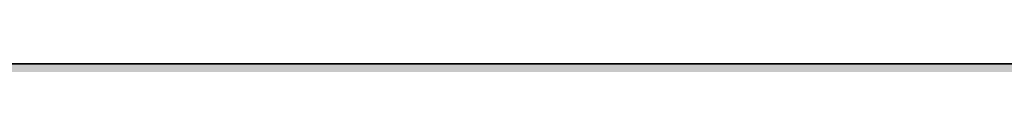
# Model space of a CAD drawing. Units: inches. Extents: x 2083 to 3317, y 1141 to 2115.
# Tile 73 of 256: x 2238.294 to 2242.452, y 1477.761 to 1477.761. Entities that reach past the tile are written whole.
import ezdxf

# ---------------------------------------------------------------- set-up
doc = ezdxf.new("R2010")
doc.units = ezdxf.units.IN
doc.layers.add('A-ANNO-DIMS', color=2, linetype='Continuous', lineweight=18)
doc.layers.add('A-WALL', color=7, linetype='Continuous', lineweight=35)
doc.layers.add('A-WALL-PATT', color=251, linetype='Continuous', lineweight=13, true_color=0x636466)
doc.styles.get("Standard").update_dxf_attribs({"font": 'arial.ttf'})
doc.dimstyles.new('ISO-25', dxfattribs={"dimtxt": 12, "dimasz": 12, "dimexe": 1.25, "dimexo": 0.625, "dimtad": 1, "dimlunit": 3, "dimtxsty": 'Standard', "dimcen": 2.5, "dimadec": 0, "dimazin": 0, "dimtfac": 1, "dimtmove": 0, "dimatfit": 3, "dimfxl": 1, "dimarcsym": 0})

# ---------------------------------------------------------------- blocks, each defined once
blk = doc.blocks.new('*D30')
at = {"layer": 'A-ANNO-DIMS', "color": 0, "lineweight": -2, "transparency": 16777216}
for p, q in [((2240.0179, 1445.2738), (2240.0179, 1448.0455)), ((2254.3293, 1445.2738), (2254.3293, 1448.0455)), ((2228.0179, 1446.7955), (2216.0179, 1446.7955)), ((2240.0179, 1446.7955), (2254.3293, 1446.7955)), ((2266.3293, 1446.7955), (2413.7649, 1446.7955))]:
    blk.add_line(p, q, dxfattribs=at)
at = {"layer": 'A-ANNO-DIMS', "color": 0, "transparency": 16777216}
for points in [[(2228.0179, 1448.7955), (2228.0179, 1444.7955), (2240.0179, 1446.7955)], [(2266.3293, 1448.7955), (2266.3293, 1444.7955), (2254.3293, 1446.7955)]]:
    blk.add_solid(points, dxfattribs=at)
at = {"layer": 'Defpoints', "color": 0, "transparency": 16777216}
for p in [(2254.3293, 1446.7955), (2240.0179, 1444.6488), (2254.3293, 1444.6488)]:
    blk.add_point(p, dxfattribs=at)
at = {"layer": 'A-ANNO-DIMS', "color": 0, "transparency": 16777216, "insert": (2346.0471, 1453.6252), "char_height": 12, "attachment_point": 5}
blk.add_mtext('WC 1\'-2 1/2" TYP.', dxfattribs=at)
blk = doc.blocks.new('*D31')
at = {"layer": 'A-ANNO-DIMS', "color": 0, "lineweight": -2, "transparency": 16777216}
for p, q in [((2237.8711, 1456.6488), (2237.8711, 1541.9152)), ((2239.3929, 1444.6488), (2236.6211, 1444.6488)), ((2237.8711, 1431.5475), (2237.8711, 1444.6488)), ((2239.3929, 1431.5475), (2236.6211, 1431.5475)), ((2237.8711, 1419.5475), (2237.8711, 1407.5475))]:
    blk.add_line(p, q, dxfattribs=at)
at = {"layer": 'A-ANNO-DIMS', "color": 0, "transparency": 16777216}
for points in [[(2235.8711, 1456.6488), (2239.8711, 1456.6488), (2237.8711, 1444.6488)], [(2235.8711, 1419.5475), (2239.8711, 1419.5475), (2237.8711, 1431.5475)]]:
    blk.add_solid(points, dxfattribs=at)
at = {"layer": 'Defpoints', "color": 0, "transparency": 16777216}
for p in [(2237.8711, 1444.6488), (2240.0179, 1444.6488), (2240.0179, 1431.5475)]:
    blk.add_point(p, dxfattribs=at)
at = {"layer": 'A-ANNO-DIMS', "color": 0, "transparency": 16777216, "insert": (2231.2175, 1505.282), "char_height": 12, "attachment_point": 5, "rotation": 90}
blk.add_mtext('1\'-1" TYP.', dxfattribs=at)
blk = doc.blocks.new('*D45')
at = {"layer": 'A-ANNO-DIMS', "color": 0, "lineweight": -2, "transparency": 16777216}
for p, q in [((2235.9598, 1478.3864), (2235.9598, 1531.3614)), ((2418.9598, 1478.3864), (2418.9598, 1531.3614)), ((2247.9598, 1530.1114), (2406.9598, 1530.1114))]:
    blk.add_line(p, q, dxfattribs=at)
at = {"layer": 'A-ANNO-DIMS', "color": 0, "transparency": 16777216}
for points in [[(2247.9598, 1532.1114), (2247.9598, 1528.1114), (2235.9598, 1530.1114)], [(2406.9598, 1532.1114), (2406.9598, 1528.1114), (2418.9598, 1530.1114)]]:
    blk.add_solid(points, dxfattribs=at)
at = {"layer": 'Defpoints', "color": 0, "transparency": 16777216}
for p in [(2418.9598, 1530.1114), (2235.9598, 1477.7614), (2418.9598, 1477.7614)]:
    blk.add_point(p, dxfattribs=at)
at = {"layer": 'A-ANNO-DIMS', "color": 0, "transparency": 16777216, "insert": (2327.4598, 1536.8673), "char_height": 12, "attachment_point": 5}
blk.add_mtext('15\'-3"', dxfattribs=at)
blk = doc.blocks.new('*D62')
at = {"layer": 'A-ANNO-DIMS', "color": 0, "lineweight": -2, "transparency": 16777216}
for p, q in [((2235.9598, 1469.3864), (2235.9598, 1522.3614)), ((2379.9598, 1469.3864), (2379.9598, 1522.3614)), ((2247.9598, 1521.1114), (2367.9598, 1521.1114))]:
    blk.add_line(p, q, dxfattribs=at)
at = {"layer": 'A-ANNO-DIMS', "color": 0, "transparency": 16777216}
for points in [[(2247.9598, 1523.1114), (2247.9598, 1519.1114), (2235.9598, 1521.1114)], [(2367.9598, 1523.1114), (2367.9598, 1519.1114), (2379.9598, 1521.1114)]]:
    blk.add_solid(points, dxfattribs=at)
at = {"layer": 'Defpoints', "color": 0, "transparency": 16777216}
for p in [(2379.9598, 1521.1114), (2235.9598, 1468.7614), (2379.9598, 1468.7614)]:
    blk.add_point(p, dxfattribs=at)
at = {"layer": 'A-ANNO-DIMS', "color": 0, "transparency": 16777216, "insert": (2307.9598, 1527.8632), "char_height": 12, "attachment_point": 5}
blk.add_mtext('12\'-0"', dxfattribs=at)

msp = doc.modelspace()

# ---------------------------------------------------------------- hatches: boundary and pattern name
at = {"layer": 'A-WALL-PATT'}
h = msp.add_hatch(color=256, dxfattribs=at)
h.dxf.hatch_style = 1
h.paths.add_polyline_path([(3126.9598, 2020.7614), (2748.9598, 2020.7614), (2604.9598, 2020.7614), (2226.9598, 2020.7614), (2226.9598, 1702.7614), (2466.9598, 1702.7614), (2466.9598, 1582.7614), (2418.9598, 1582.7614), (2418.9598, 1477.7614), (2226.9598, 1477.7614), (2226.9598, 1263.2614), (2544.9598, 1263.2614), (2544.9598, 1411.7614), (2604.9598, 1411.7614), (2685.9598, 1411.7614), (2685.9598, 1420.7614), (2604.9598, 1420.7614), (2604.9598, 1573.7614), (2604.9598, 1702.7614), (2604.9598, 2011.7614), (2748.9598, 2011.7614), (2748.9598, 1702.7614), (2862.9598, 1702.7614), (2862.9598, 1621.7614), (2871.9598, 1621.7614), (2871.9598, 1702.7614), (2883.9598, 1702.7614), (2883.9598, 1706.9395, -0.026459), (2883.9598, 1711.7614), (2757.9598, 1711.7614), (2757.9598, 1807.7614), (2787.9598, 1807.7614), (2787.9598, 1812.2614), (2757.9598, 1812.2614), (2757.9598, 2011.7614), (2877.9598, 2011.7614), (2877.9598, 1812.2614), (2847.9598, 1812.2614), (2847.9598, 1807.7614), (2889.8357, 1807.7614), (2889.8357, 1812.2614), (2882.4598, 1812.2614), (2882.4598, 2011.7614), (3117.9598, 2011.7614), (3117.9598, 1812.2614), (2937.8357, 1812.2614), (2937.8357, 1807.7614), (2995.7098, 1807.7614), (2995.7098, 1796.1177), (3000.2098, 1796.1177), (3000.2098, 1807.7614), (3117.9598, 1807.7614), (3117.9598, 1711.7614), (3000.2098, 1711.7614), (3000.2098, 1760.1177), (2998.5727, 1760.1177, -0.020711), (2995.7098, 1760.1177), (2995.7098, 1711.7614), (2931.9598, 1711.7614), (2931.9598, 1702.7614), (3126.9598, 1702.7614)])
h.paths.add_polyline_path([(2471.4598, 2011.7614), (2471.4598, 1810.0114), (2462.7169, 1810.0114), (2462.7169, 1805.5114), (2505.9598, 1805.5114), (2505.9598, 1810.0114), (2475.9598, 1810.0114), (2475.9598, 2011.7614), (2595.9598, 2011.7614), (2595.9598, 1810.0114), (2565.9598, 1810.0114), (2565.9598, 1805.5114), (2595.9598, 1805.5114), (2595.9598, 1711.7614), (2235.9598, 1711.7614), (2235.9598, 1805.5114), (2353.7098, 1805.5114), (2353.7098, 1796.0542), (2358.2098, 1796.0542), (2358.2098, 1805.5114), (2414.7169, 1805.5114), (2414.7169, 1810.0114), (2235.9598, 1810.0114), (2235.9598, 2011.7614)], flags=16)
h.paths.add_polyline_path([(2270.2047, 1994.61), (2270.2047, 1970.61), (2246.2047, 1970.61), (2246.2047, 1994.61)], flags=0)
edge = h.paths.add_edge_path(flags=0)
edge.add_ellipse((2332.0274, 1899.7982), major_axis=(-3.043, 3.043), ratio=0.168252, start_angle=-161.3322, end_angle=-156.3071, ccw=False)
edge.add_ellipse((2333.082, 1898.7435), major_axis=(-1.0546, 1.0546), ratio=0.453532, start_angle=-123.371, end_angle=-94.1591)
edge = h.paths.add_edge_path(flags=0)
edge.add_ellipse((2332.0274, 1968.8763), major_axis=(3.043, 3.043), ratio=0.168252, start_angle=18.6678, end_angle=23.6929)
edge.add_spline(control_points=[(2332.9256, 1970.6911), (2332.2268, 1970.3361), (2330.8937, 1969.6589), (2328.4131, 1970.9321), (2327.2039, 1967.7487), (2324.7096, 1969.9556), (2322.5328, 1967.0124), (2320.0128, 1971.2958), (2317.6803, 1968.1578), (2316.0405, 1967.102), (2315.4269, 1966.8096)], knot_values=[0, 0, 0, 0, 2.267059, 4.324559, 6.685584, 8.878641, 11.121502, 14.300359, 17.755284, 19.732645, 19.732645, 19.732645, 19.732645], degree=3, periodic=0)
edge.add_ellipse((2332.0274, 1968.8763), major_axis=(3.043, 3.043), ratio=0.168252, start_angle=18.6678, end_angle=23.6929, ccw=False)
edge.add_ellipse((2333.082, 1969.9309), major_axis=(1.0546, 1.0546), ratio=0.453532, start_angle=56.629, end_angle=85.8409, ccw=False)
edge = h.paths.add_edge_path(flags=0)
edge.add_spline(control_points=[(2296.4283, 1967.9879), (2293.6278, 1965.3363), (2287.7036, 1959.7271), (2299.7439, 1949.9957), (2294.5326, 1935.6685), (2290.5732, 1920.6035), (2293.3941, 1909.9737), (2296.1854, 1904.9665)], knot_values=[0.099185, 0.099185, 0.099185, 0.099185, 0.345301, 0.619822, 0.982653, 1.386093, 1.810555, 1.810555, 1.810555, 1.810555], degree=3, periodic=0)
edge.add_spline(control_points=[(2296.1854, 1904.9665), (2297.3836, 1902.6193), (2298.001, 1901.9493), (2298.553, 1901.4682)], knot_values=[0.006246, 0.006246, 0.006246, 0.006246, 0.055476, 0.055476, 0.055476, 0.055476], degree=3, periodic=0)
edge.add_spline(control_points=[(2298.553, 1901.4682), (2297.2586, 1900.9232), (2295.2253, 1900.2321), (2293.0602, 1900.6142), (2292.1014, 1900.7884), (2292.0896, 1900.7906)], knot_values=[0.312835, 0.312835, 0.312835, 0.312835, 0.40178, 0.474987, 0.475903, 0.475903, 0.475903, 0.475903], degree=3, periodic=0)
edge.add_arc((2292.7936, 1904.6641), 3.937, 215.4209, 259.6982, ccw=False)
edge.add_spline(control_points=[(2289.5853, 1902.3823), (2289.4767, 1902.5351), (2289.3685, 1902.688), (2289.2609, 1902.8412)], knot_values=[0.102872, 0.102872, 0.102872, 0.102872, 0.116896, 0.116896, 0.116896, 0.116896], degree=3, periodic=0)
edge.add_spline(control_points=[(2289.2609, 1902.8412), (2288.6866, 1902.5502), (2287.64, 1902.0199), (2285.8813, 1901.874), (2283.853, 1901.5044), (2281.72, 1899.7105), (2278.467, 1899.4929), (2276.1571, 1901.8832), (2272.259, 1899.8041), (2267.7776, 1901.8432), (2262.2439, 1900.184), (2257.4149, 1901.7821), (2254.3184, 1900.7261), (2253.1783, 1900.3373)], knot_values=[0, 0, 0, 0, 1.907977, 3.477176, 5.261074, 7.972851, 11.680248, 13.717921, 16.939592, 22.789562, 27.502503, 33.595215, 37.145618, 37.145618, 37.145618, 37.145618], degree=3, periodic=0)
edge.add_line((2253.1783, 1900.3373), (2250.2442, 1902.8412))
edge.add_line((2250.2442, 1902.8412), (2250.2442, 1965.8333))
edge.add_line((2250.2442, 1965.8333), (2253.1783, 1968.3371))
edge.add_spline(control_points=[(2253.1783, 1968.3371), (2254.3184, 1967.9483), (2257.4149, 1966.8924), (2262.2439, 1968.4904), (2267.7776, 1966.8313), (2271.5267, 1968.5372), (2273.8759, 1967.8283), (2274.2067, 1967.7276)], knot_values=[0, 0, 0, 0, 0.09018, 0.244935, 0.364644, 0.513233, 0.537855, 0.537855, 0.537855, 0.537855], degree=3, periodic=0)
edge.add_arc((2274.3529, 1963.7933), 3.937, 72.0511, 92.1279, ccw=False)
edge.add_arc((2281.2969, 1985.23), 18.5963, 252.05113, 288.56572)
edge.add_arc((2292.3167, 1956.0289), 12.6461, 71.02679, 113.77822, ccw=False)
edge = h.paths.add_edge_path(flags=0)
edge.add_spline(control_points=[(2274.8994, 1951.8562), (2275.0662, 1951.6166), (2275.2327, 1951.3766), (2275.398, 1951.1359)], knot_values=[1.409916, 1.409916, 1.409916, 1.409916, 1.43159, 1.43159, 1.43159, 1.43159], degree=3, periodic=0)
edge.add_spline(control_points=[(2275.398, 1951.1359), (2275.7921, 1950.5619), (2276.1792, 1949.9838), (2276.5455, 1949.3971)], knot_values=[1.358238, 1.358238, 1.358238, 1.358238, 1.409916, 1.409916, 1.409916, 1.409916], degree=3, periodic=0)
edge.add_line((2276.5455, 1949.3971), (2277.4373, 1947.8622))
edge.add_spline(control_points=[(2277.4373, 1947.8622), (2276.3038, 1945.6731), (2274.6397, 1942.4269), (2274.6316, 1938.0939), (2272.7991, 1930.8515), (2274.3564, 1943.897), (2275.9477, 1947.9234), (2276.5455, 1949.3971)], knot_values=[0.005632, 0.005632, 0.005632, 0.005632, 0.186014, 0.266002, 0.357087, 0.59639, 0.739732, 0.739732, 0.739732, 0.739732], degree=3, periodic=0)
edge.add_spline(control_points=[(2276.5455, 1949.3971), (2276.1792, 1949.9838), (2275.7921, 1950.5619), (2275.398, 1951.1359)], knot_values=[1.358238, 1.358238, 1.358238, 1.358238, 1.409916, 1.409916, 1.409916, 1.409916], degree=3, periodic=0)
edge.add_spline(control_points=[(2275.398, 1951.1359), (2274.9425, 1950.0805), (2274.2078, 1948.0253), (2273.9346, 1944.8515), (2272.4685, 1937.6275), (2273.4662, 1945.6965), (2274.7006, 1951.0595), (2274.8994, 1951.8562)], knot_values=[0.104364, 0.104364, 0.104364, 0.104364, 0.189636, 0.269624, 0.36071, 0.600013, 0.644622, 0.644622, 0.644622, 0.644622], degree=3, periodic=0)
h.paths.add_polyline_path([(2269.1675, 1963.1276, -0.357527), (2268.1706, 1960.9764, -0.092561), (2268.1706, 1939.4363, -0.357527), (2269.1675, 1937.2851, -0.357527), (2267.0163, 1938.282, -0.164785), (2254.6856, 1938.282, -0.357527), (2252.5344, 1937.2851, -0.357527), (2253.5313, 1939.4363, -0.092561), (2253.5313, 1960.9764, -0.357527), (2252.5344, 1963.1276, -0.357527), (2254.6856, 1962.1307, -0.164785), (2267.0163, 1962.1307, -0.357527)], flags=0)
h.paths.add_polyline_path([(2248.8741, 1967.8018), (2248.8741, 1957.0277), (2249.4578, 1957.0277), (2249.4578, 1911.6468), (2248.8741, 1911.6468), (2248.8741, 1900.8727), (2246.5119, 1900.8727, 0.197327), (2244.1497, 1902.4569), (2244.1497, 1966.2176, 0.197327), (2246.5119, 1967.8018)], flags=0)
h.paths.add_polyline_path([(2269.1675, 1931.3893, -0.357527), (2268.1706, 1929.2381, -0.092561), (2268.1706, 1907.6981, -0.357527), (2269.1675, 1905.5469, -0.357527), (2267.0163, 1906.5438, -0.164785), (2254.6856, 1906.5438, -0.357527), (2252.5344, 1905.5469, -0.357527), (2253.5313, 1907.6981, -0.092561), (2253.5313, 1929.2381, -0.357527), (2252.5344, 1931.3893, -0.357527), (2254.6856, 1930.3925, -0.164785), (2267.0163, 1930.3925, -0.357527)], flags=0)
edge = h.paths.add_edge_path(flags=0)
edge.add_spline(control_points=[(2276.1969, 1906.7237), (2276.1681, 1909.0289), (2276.114, 1913.3719), (2270.5984, 1924.925), (2273.9052, 1919.0128), (2275.9217, 1916.2621), (2275.4746, 1912.4021), (2277.2579, 1910.3806), (2276.696, 1908.225), (2276.6462, 1906.813), (2276.6178, 1906.0084)], knot_values=[0, 0, 0, 0, 8.61026, 16.221274, 18.843057, 23.804898, 27.440828, 29.356102, 31.203478, 33.650687, 33.650687, 33.650687, 33.650687], degree=3, periodic=0)
edge.add_spline(control_points=[(2276.6178, 1906.0084), (2276.6233, 1905.6241), (2276.4977, 1904.6287), (2275.4418, 1903.8547), (2274.9373, 1903.0804), (2274.8591, 1902.8412)], knot_values=[0.156488, 0.156488, 0.156488, 0.156488, 0.184398, 0.231376, 0.250598, 0.250598, 0.250598, 0.250598], degree=3, periodic=0)
edge.add_line((2274.8591, 1902.8412), (2276.506, 1902.8412))
edge.add_spline(control_points=[(2276.506, 1902.8412), (2276.7883, 1903.0849), (2277.6651, 1904.1252), (2278.2495, 1904.3407), (2277.6539, 1908.5274), (2278.1557, 1906.2278), (2278.1005, 1905.2859), (2278.8467, 1904.069), (2277.8568, 1903.4149), (2277.8742, 1902.991), (2277.9036, 1902.8412)], knot_values=[0.059574, 0.059574, 0.059574, 0.059574, 0.080753, 0.103741, 0.16972, 0.176036, 0.207137, 0.240474, 0.262341, 0.27366, 0.27366, 0.27366, 0.27366], degree=3, periodic=0)
edge.add_line((2277.9036, 1902.8412), (2280.0298, 1902.8412))
edge.add_spline(control_points=[(2280.0298, 1902.8412), (2279.8882, 1903.0884), (2279.4993, 1903.9816), (2280.1523, 1905.9393), (2278.1036, 1909.6578), (2279.7624, 1907.1853), (2280.3279, 1904.8749), (2280.4851, 1903.4896), (2281.4633, 1903.2494), (2281.7583, 1902.9365), (2281.834, 1902.8412)], knot_values=[0.013856, 0.013856, 0.013856, 0.013856, 0.034874, 0.088867, 0.107879, 0.126738, 0.158714, 0.193757, 0.217487, 0.226722, 0.226722, 0.226722, 0.226722], degree=3, periodic=0)
edge.add_spline(control_points=[(2281.834, 1902.8412), (2281.7875, 1902.8267), (2281.647, 1902.783), (2281.3955, 1902.8595), (2281.0881, 1902.9852), (2280.7207, 1903.0609), (2280.3335, 1903.0257), (2280.1248, 1902.8989), (2280.0298, 1902.8412)], knot_values=[0, 0, 0, 0, 0.14413, 0.435517, 0.749276, 1.153046, 1.548371, 1.878348, 1.878348, 1.878348, 1.878348], degree=3, periodic=0)
edge.add_line((2280.0298, 1902.8412), (2277.9036, 1902.8412))
edge.add_spline(control_points=[(2277.9036, 1902.8412), (2277.8929, 1902.7959), (2277.8654, 1902.6796), (2277.6075, 1902.6875), (2277.2741, 1902.8007), (2276.8379, 1902.6198), (2276.5838, 1902.7893), (2276.506, 1902.8412)], knot_values=[0, 0, 0, 0, 0.127189, 0.326199, 0.628009, 1.24357, 1.515331, 1.515331, 1.515331, 1.515331], degree=3, periodic=0)
edge.add_line((2276.506, 1902.8412), (2274.8591, 1902.8412))
edge.add_spline(control_points=[(2274.8591, 1902.8412), (2274.8144, 1902.8986), (2274.7251, 1903.0134), (2274.4935, 1903.119), (2274.2443, 1902.9605), (2273.9371, 1903.1849), (2273.614, 1902.9831), (2273.4083, 1902.883), (2273.3223, 1902.8412)], knot_values=[0, 0, 0, 0, 0.21843, 0.436957, 0.687977, 0.990379, 1.398396, 1.69185, 1.69185, 1.69185, 1.69185], degree=3, periodic=0)
edge.add_spline(control_points=[(2273.3223, 1902.8412), (2273.6167, 1903.4457), (2274.274, 1904.5383), (2276.0272, 1904.5737), (2276.207, 1906.5836), (2276.1969, 1906.7237)], knot_values=[0.012227, 0.012227, 0.012227, 0.012227, 0.059472, 0.106218, 0.134458, 0.134458, 0.134458, 0.134458], degree=3, periodic=0)
h.paths.add_polyline_path([(2270.7761, 1897.7898), (2270.7761, 1873.7898), (2246.7761, 1873.7898), (2246.7761, 1897.7898)], flags=0)
h.paths.add_polyline_path([(2353.7098, 1760.0051), (2353.7098, 1760.0542), (2358.2098, 1760.0542, -0.033729)], flags=0)
h.paths.add_polyline_path([(2321.8191, 1737.5292), (2341.9953, 1737.5292, -0.414214), (2343.2033, 1736.3212), (2343.2033, 1721.0206, -0.414214), (2341.9953, 1719.8127), (2321.8191, 1719.8127, -0.414214), (2320.6112, 1721.0206), (2320.6112, 1736.3212, -0.414214)], flags=0)
h.paths.add_polyline_path([(2324.235, 1736.3212), (2339.5794, 1736.3212, -0.414214), (2341.9953, 1733.9053), (2341.9953, 1725.4497, -0.414214), (2339.5794, 1723.0338), (2333.6806, 1723.0338), (2333.8453, 1722.0455, -0.870646), (2335.4254, 1721.8259, -0.767327), (2333.9227, 1721.4232), (2331.291, 1721.4232, -0.767327), (2329.7883, 1721.8259, -0.870646), (2331.3684, 1722.0455), (2331.5331, 1723.0338), (2324.235, 1723.0338, -0.414214), (2321.8191, 1725.4497), (2321.8191, 1733.9053, -0.414214)], flags=0)
h.paths.add_polyline_path([(2570.4838, 1928.6154), (2589.6838, 1928.6154), (2590.1688, 1928.6154), (2590.1688, 1904.9934), (2570.4838, 1904.9934)], flags=0)
h.paths.add_polyline_path([(2574.4473, 1927.2638, -1), (2572.8288, 1927.2638, -1)], flags=0)
h.paths.add_polyline_path([(2573.0899, 1926.9409), (2573.925, 1927.776), (2574.1477, 1927.5533), (2573.3126, 1926.7182)], flags=0)
h.paths.add_polyline_path([(2578.7791, 1919.7296, -1), (2571.5917, 1919.7296, -1)], flags=0)
h.paths.add_polyline_path([(2578.3854, 1919.7296, -1), (2571.9854, 1919.7296, -1)], flags=0)
h.paths.add_polyline_path([(2331.5958, 1729.4762, -1), (2333.618, 1729.4762, -1)], flags=0)
h.paths.add_polyline_path([(2578.0342, 1927.2638, -1), (2576.4157, 1927.2638, -1)], flags=0)
h.paths.add_polyline_path([(2576.6889, 1927.5311), (2576.9116, 1927.7538), (2577.7467, 1926.9186), (2577.524, 1926.6959)], flags=0)
h.paths.add_polyline_path([(2578.1391, 1909.8595, -1), (2572.2317, 1909.8595, -1)], flags=0)
h.paths.add_polyline_path([(2577.7454, 1909.8595, -1), (2572.6254, 1909.8595, -1)], flags=0)
h.paths.add_polyline_path([(2583.7977, 1927.2638, -1), (2582.1792, 1927.2638, -1)], flags=0)
h.paths.add_polyline_path([(2582.7186, 1927.7538), (2583.5538, 1926.9186), (2583.3311, 1926.6959), (2582.4959, 1927.5311)], flags=0)
h.paths.add_polyline_path([(2582.4959, 1927.5311), (2582.7186, 1927.7538), (2583.5538, 1926.9186), (2583.3311, 1926.6959)], flags=0)
h.paths.add_polyline_path([(2587.7391, 1920.5296, -1), (2581.8317, 1920.5296, -1)], flags=0)
h.paths.add_polyline_path([(2587.3454, 1920.5296, -1), (2582.2254, 1920.5296, -1)], flags=0)
h.paths.add_polyline_path([(2587.3846, 1927.2638, -1), (2585.7661, 1927.2638, -1)], flags=0)
h.paths.add_polyline_path([(2586.082, 1926.9802), (2586.9172, 1927.8154), (2587.1399, 1927.5927), (2586.3047, 1926.7575)], flags=0)
h.paths.add_polyline_path([(2588.3791, 1910.6595, -1), (2581.1917, 1910.6595, -1)], flags=0)
h.paths.add_polyline_path([(2587.9854, 1910.6595, -1), (2581.5854, 1910.6595, -1)], flags=0)
h.paths.add_polyline_path([(2417.1677, 1729.4779), (2437.3439, 1729.4779, -0.414214), (2438.5519, 1728.2699), (2438.5519, 1712.9693, -0.414214), (2437.3439, 1711.7614), (2417.1677, 1711.7614, -0.414214), (2415.9598, 1712.9693), (2415.9598, 1728.2699, -0.414214)], flags=0)
h.paths.add_polyline_path([(2419.5836, 1728.2699), (2434.928, 1728.2699, -0.414214), (2437.3439, 1725.8541), (2437.3439, 1717.3984, -0.414214), (2434.928, 1714.9825), (2429.0292, 1714.9825), (2429.1939, 1713.9942, -0.870646), (2430.774, 1713.7746, -0.767327), (2429.2713, 1713.372), (2426.6396, 1713.372, -0.767327), (2425.1369, 1713.7746, -0.870646), (2426.717, 1713.9942), (2426.8817, 1714.9825), (2419.5836, 1714.9825, -0.414214), (2417.1677, 1717.3984), (2417.1677, 1725.8541, -0.414214)], flags=0)
h.paths.add_polyline_path([(2419.5836, 1728.2699), (2434.928, 1728.2699, -0.414214), (2437.3439, 1725.8541), (2437.3439, 1717.3984, -0.414214), (2434.928, 1714.9825), (2429.0292, 1714.9825), (2428.3581, 1719.009), (2427.5528, 1719.009), (2426.8817, 1714.9825), (2419.5836, 1714.9825, -0.414214), (2417.1677, 1717.3984), (2417.1677, 1725.8541, -0.414214)], flags=0)
h.paths.add_polyline_path([(2426.9444, 1721.4249, -1), (2428.9666, 1721.4249, -1)], flags=0)
h.paths.add_polyline_path([(2475.9598, 1702.7614), (2595.9598, 1702.7614), (2595.9598, 1582.7614), (2475.9598, 1582.7614)], flags=16)
h.paths.add_polyline_path([(2427.9598, 1573.7614), (2595.9598, 1573.7614), (2595.9598, 1468.7614), (2595.9598, 1420.7614), (2384.4598, 1420.7614), (2384.4598, 1468.7614), (2427.9598, 1468.7614)], flags=16)
h.paths.add_polyline_path([(2379.9598, 1468.7614), (2379.9598, 1420.7614), (2235.9598, 1420.7614), (2235.9598, 1468.7614)], flags=16)
h.paths.add_polyline_path([(2317.816, 1466.6958), (2337.9922, 1466.6958, -0.414214), (2339.2002, 1465.4878), (2339.2002, 1450.1872, -0.414214), (2337.9922, 1448.9792), (2317.816, 1448.9792, -0.414214), (2316.6081, 1450.1872), (2316.6081, 1465.4878, -0.414214)], flags=0)
h.paths.add_polyline_path([(2320.2319, 1465.4878), (2335.5763, 1465.4878, -0.414214), (2337.9922, 1463.0719), (2337.9922, 1454.6163, -0.414214), (2335.5763, 1452.2004), (2329.6775, 1452.2004), (2329.8422, 1451.212, -0.870646), (2331.4223, 1450.9925, -0.767327), (2329.9196, 1450.5898), (2327.2879, 1450.5898, -0.767327), (2325.7852, 1450.9925, -0.870646), (2327.3653, 1451.212), (2327.53, 1452.2004), (2320.2319, 1452.2004, -0.414214), (2317.816, 1454.6163), (2317.816, 1463.0719, -0.414214)], flags=0)
h.paths.add_polyline_path([(2320.2319, 1465.4878), (2335.5763, 1465.4878, -0.414214), (2337.9922, 1463.0719), (2337.9922, 1454.6163, -0.414214), (2335.5763, 1452.2004), (2329.6775, 1452.2004), (2329.0064, 1456.2269), (2328.2011, 1456.2269), (2327.53, 1452.2004), (2320.2319, 1452.2004, -0.414214), (2317.816, 1454.6163), (2317.816, 1463.0719, -0.414214)], flags=0)
h.paths.add_polyline_path([(2327.5926, 1458.6428, -1), (2329.6148, 1458.6428, -1)], flags=0)
h.paths.add_polyline_path([(2244.4117, 1433.3405), (2241.9209, 1433.3405, -0.414214), (2240.0179, 1435.2435), (2240.0179, 1440.9528, -0.414211), (2241.9209, 1442.8559), (2244.4117, 1442.8559, -1.976472)], flags=0)
h.paths.add_polyline_path([(2245.3569, 1434.3975, -0.414214), (2245.3569, 1441.7988, -2.144098)], flags=0)
h.paths.add_polyline_path([(2535.9598, 1416.2614), (2535.9598, 1272.2614), (2235.9598, 1272.2614), (2235.9598, 1416.2614)], flags=16)
h.paths.add_polyline_path([(2260.1196, 1384.2928), (2260.1196, 1362.0386), (2237.8654, 1362.0386), (2237.8654, 1384.2928)], flags=0)
edge = h.paths.add_edge_path(flags=0)
edge.add_line((2318.2518, 1362.0933), (2318.1458, 1362.001))
edge.add_ellipse((2317.4451, 1360.431), major_axis=(2.8216, 2.8216), ratio=0.168252, start_angle=18.6678, end_angle=20.9481, ccw=False)
edge.add_ellipse((2318.423, 1361.409), major_axis=(0.9779, 0.9779), ratio=0.453532, start_angle=56.629, end_angle=70.2262, ccw=False)
edge = h.paths.add_edge_path(flags=0)
edge.add_line((2319.1074, 1295.5711), (2319.015, 1295.6771))
edge.add_ellipse((2317.4451, 1296.3778), major_axis=(-2.8216, 2.8216), ratio=0.168252, start_angle=-161.3322, end_angle=-159.0519, ccw=False)
edge.add_ellipse((2318.423, 1295.3999), major_axis=(-0.9779, 0.9779), ratio=0.453532, start_angle=-123.371, end_angle=-109.7738)
edge = h.paths.add_edge_path(flags=0)
edge.add_spline(control_points=[(2284.2103, 1301.1702), (2284.5807, 1300.4447), (2284.8912, 1299.892), (2285.1596, 1299.461)], knot_values=[0.039066, 0.039066, 0.039066, 0.039066, 0.055476, 0.055476, 0.055476, 0.055476], degree=3, periodic=0)
edge.add_line((2285.1596, 1299.461), (2284.2103, 1301.1702))
edge = h.paths.add_edge_path(flags=0)
edge.add_line((2280.4125, 1297.298), (2283.37, 1297.0361))
edge.add_line((2283.37, 1297.0361), (2286.4057, 1297.9263))
edge.add_spline(control_points=[(2286.4057, 1297.9263), (2285.3055, 1297.4631), (2284.3448, 1297.1292), (2283.37, 1297.0361)], knot_values=[0.394369, 0.394369, 0.394369, 0.394369, 0.475903, 0.475903, 0.475903, 0.475903], degree=3, periodic=0)
edge.add_spline(control_points=[(2283.37, 1297.0361), (2283.2814, 1297.0277), (2282.3163, 1296.9573), (2281.3125, 1297.1345), (2280.4234, 1297.296), (2280.4125, 1297.298)], knot_values=[0.312835, 0.312835, 0.312835, 0.312835, 0.320246, 0.393453, 0.394369, 0.394369, 0.394369, 0.394369], degree=3, periodic=0)
edge = h.paths.add_edge_path(flags=0)
edge.add_line((2284.4356, 1359.6073), (2280.4463, 1355.328))
edge.add_line((2280.4463, 1355.328), (2279.58, 1351.0178))
edge.add_line((2279.58, 1351.0178), (2282.413, 1346.5804))
edge.add_spline(control_points=[(2282.413, 1346.5804), (2283.1533, 1345.5892), (2284.2529, 1344.0289), (2284.801, 1342.3872), (2284.9352, 1341.8055)], knot_values=[1.240098, 1.240098, 1.240098, 1.240098, 1.332892, 1.382712, 1.382712, 1.382712, 1.382712], degree=3, periodic=0)
edge.add_spline(control_points=[(2284.9352, 1341.8055), (2285.3191, 1340.1406), (2285.233, 1338.4092), (2284.9099, 1336.6541)], knot_values=[1.097484, 1.097484, 1.097484, 1.097484, 1.240098, 1.240098, 1.240098, 1.240098], degree=3, periodic=0)
edge.add_spline(control_points=[(2284.9099, 1336.6541), (2284.5868, 1334.899), (2284.0267, 1333.1203), (2283.4626, 1331.3606)], knot_values=[0.95487, 0.95487, 0.95487, 0.95487, 1.097484, 1.097484, 1.097484, 1.097484], degree=3, periodic=0)
edge.add_line((2283.4626, 1331.3606), (2281.8904, 1326.1534))
edge.add_line((2281.8904, 1326.1534), (2280.7563, 1321.0561))
edge.add_line((2280.7563, 1321.0561), (2280.2992, 1316.002))
edge.add_line((2280.2992, 1316.002), (2280.7159, 1310.9501))
edge.add_line((2280.7159, 1310.9501), (2282.0281, 1305.9721))
edge.add_line((2282.0281, 1305.9721), (2284.2103, 1301.1702))
edge.add_spline(control_points=[(2284.2103, 1301.1702), (2283.3407, 1302.7302), (2282.6119, 1304.3365), (2282.0281, 1305.9721)], knot_values=[0.099185, 0.099185, 0.099185, 0.099185, 0.241799, 0.241799, 0.241799, 0.241799], degree=3, periodic=0)
edge.add_spline(control_points=[(2282.0281, 1305.9721), (2281.4443, 1307.6078), (2281.0055, 1309.2728), (2280.7159, 1310.9501)], knot_values=[0.241799, 0.241799, 0.241799, 0.241799, 0.384413, 0.384413, 0.384413, 0.384413], degree=3, periodic=0)
edge.add_spline(control_points=[(2280.7159, 1310.9501), (2280.4332, 1312.5876), (2280.2894, 1314.277), (2280.2989, 1315.962), (2280.2992, 1316.002)], knot_values=[0.384413, 0.384413, 0.384413, 0.384413, 0.523647, 0.527028, 0.527028, 0.527028, 0.527028], degree=3, periodic=0)
edge.add_spline(control_points=[(2280.2992, 1316.002), (2280.3123, 1317.687), (2280.4779, 1319.3679), (2280.7563, 1321.0561)], knot_values=[0.527028, 0.527028, 0.527028, 0.527028, 0.669642, 0.669642, 0.669642, 0.669642], degree=3, periodic=0)
edge.add_spline(control_points=[(2280.7563, 1321.0561), (2281.0346, 1322.7443), (2281.4259, 1324.4396), (2281.8904, 1326.1534)], knot_values=[0.669642, 0.669642, 0.669642, 0.669642, 0.812256, 0.812256, 0.812256, 0.812256], degree=3, periodic=0)
edge.add_spline(control_points=[(2281.8904, 1326.1534), (2282.2644, 1327.5333), (2282.7879, 1329.2618), (2283.3528, 1331.0178), (2283.4626, 1331.3606)], knot_values=[0.812256, 0.812256, 0.812256, 0.812256, 0.927087, 0.95487, 0.95487, 0.95487, 0.95487], degree=3, periodic=0)
edge.add_line((2283.4626, 1331.3606), (2284.9099, 1336.6541))
edge.add_line((2284.9099, 1336.6541), (2284.9352, 1341.8055))
edge.add_line((2284.9352, 1341.8055), (2282.413, 1346.5804))
edge.add_spline(control_points=[(2282.413, 1346.5804), (2281.2751, 1348.1038), (2280.0784, 1349.5703), (2279.58, 1351.0178)], knot_values=[1.382712, 1.382712, 1.382712, 1.382712, 1.525326, 1.525326, 1.525326, 1.525326], degree=3, periodic=0)
edge.add_spline(control_points=[(2279.58, 1351.0178), (2279.4433, 1351.4147), (2279.1363, 1352.8569), (2279.7352, 1354.2904), (2280.4463, 1355.328)], knot_values=[1.525326, 1.525326, 1.525326, 1.525326, 1.564439, 1.667941, 1.667941, 1.667941, 1.667941], degree=3, periodic=0)
edge.add_spline(control_points=[(2280.4463, 1355.328), (2281.4261, 1356.7578), (2282.9308, 1358.1826), (2284.4356, 1359.6073)], knot_values=[1.667941, 1.667941, 1.667941, 1.667941, 1.810555, 1.810555, 1.810555, 1.810555], degree=3, periodic=0)
edge.add_arc((2280.6231, 1348.5182), 11.7262, 71.02679, 113.77822)
edge.add_arc((2270.4049, 1375.5952), 17.2436, 252.05113, 288.56572, ccw=False)
edge.add_arc((2263.966, 1355.7178), 3.6506, 72.0511, 92.1279)
edge.add_arc((2263.966, 1355.7178), 3.6506, 92.1279, 177.9851)
edge.add_spline(control_points=[(2260.3176, 1355.8462), (2260.2604, 1354.2207), (2260.5513, 1350.1865), (2262.9993, 1346.7663), (2264.4727, 1344.649)], knot_values=[1.43159, 1.43159, 1.43159, 1.43159, 1.564144, 1.770695, 1.770695, 1.770695, 1.770695], degree=3, periodic=0)
edge.add_line((2264.4727, 1344.649), (2264.9356, 1343.9825))
edge.add_spline(control_points=[(2263.801, 1340.2481), (2263.8432, 1340.5141), (2264.0672, 1341.7565), (2264.5127, 1343.0025), (2264.935, 1343.9811)], knot_values=[0.53657, 0.53657, 0.53657, 0.53657, 0.559349, 0.644622, 0.644622, 0.644622, 0.644622], degree=3, periodic=0)
edge.add_spline(control_points=[(2264.935, 1343.9811), (2265.1178, 1343.715), (2265.2989, 1343.4479), (2265.4768, 1343.1794)], knot_values=[1.384077, 1.384077, 1.384077, 1.384077, 1.409916, 1.409916, 1.409916, 1.409916], degree=3, periodic=0)
edge.add_spline(control_points=[(2265.4768, 1343.1794), (2265.6546, 1342.9108), (2265.8293, 1342.6408), (2265.9991, 1342.3688)], knot_values=[1.358238, 1.358238, 1.358238, 1.358238, 1.384077, 1.384077, 1.384077, 1.384077], degree=3, periodic=0)
edge.add_line((2265.9991, 1342.3688), (2266.826, 1340.9455))
edge.add_spline(control_points=[(2266.826, 1340.9455), (2268.8944, 1337.0897), (2271.3982, 1325.843), (2270.5162, 1310.5686), (2275.9194, 1301.8606), (2277.7895, 1299.1994)], knot_values=[0.116896, 0.116896, 0.116896, 0.116896, 0.472987, 1.050969, 1.313793, 1.313793, 1.313793, 1.313793], degree=3, periodic=0)
edge.add_spline(control_points=[(2277.7895, 1299.1994), (2277.8394, 1299.1285), (2277.8894, 1299.0575), (2277.9396, 1298.9866)], knot_values=[0.109884, 0.109884, 0.109884, 0.109884, 0.116896, 0.116896, 0.116896, 0.116896], degree=3, periodic=0)
edge.add_line((2277.9396, 1298.9866), (2277.7888, 1299.1991))
edge.add_spline(control_points=[(2277.7888, 1299.1991), (2277.2566, 1298.9294), (2276.2864, 1298.4379), (2275.0394, 1298.3344), (2274.3833, 1298.2389), (2274.2153, 1298.2093)], knot_values=[33.12187, 33.12187, 33.12187, 33.12187, 35.029056, 36.598255, 37.144827, 37.144827, 37.144827, 37.144827], degree=3, periodic=0)
edge.add_line((2274.2153, 1298.2093), (2273.0731, 1297.893))
edge.add_spline(control_points=[(2273.0731, 1297.893), (2272.3229, 1297.5798), (2271.0392, 1296.5105), (2269.2484, 1296.2261), (2268.4231, 1296.3747)], knot_values=[26.532584, 26.532584, 26.532584, 26.532584, 29.198919, 31.839101, 31.839101, 31.839101, 31.839101], degree=3, periodic=0)
edge.add_line((2268.4231, 1296.3747), (2263.8785, 1297.4575))
edge.add_spline(control_points=[(2263.8785, 1297.4575), (2263.5561, 1297.3594), (2261.8603, 1296.8387), (2260.2388, 1297.2824), (2258.9335, 1297.5165)], knot_values=[15.919551, 15.919551, 15.919551, 15.919551, 16.939592, 21.226067, 21.226067, 21.226067, 21.226067], degree=3, periodic=0)
edge.add_line((2258.9335, 1297.5165), (2254.0552, 1297.329))
edge.add_spline(control_points=[(2254.0552, 1297.329), (2253.7555, 1297.2958), (2252.1137, 1297.1652), (2250.4619, 1297.5442), (2249.1297, 1297.6679)], knot_values=[5.306517, 5.306517, 5.306517, 5.306517, 6.276435, 10.613034, 10.613034, 10.613034, 10.613034], degree=3, periodic=0)
edge.add_line((2249.1297, 1297.6679), (2244.3316, 1296.8778))
edge.add_line((2244.3316, 1296.8778), (2241.611, 1299.1994))
edge.add_line((2241.611, 1299.1994), (2241.611, 1357.6094))
edge.add_line((2241.611, 1357.6094), (2244.3316, 1359.9311))
edge.add_line((2244.3316, 1359.9311), (2252.7288, 1359.5427))
edge.add_spline(control_points=[(2252.7288, 1359.5427), (2252.8709, 1359.5464), (2253.3057, 1359.5482), (2253.7398, 1359.5143), (2254.0317, 1359.4824)], knot_values=[0.233291, 0.233291, 0.233291, 0.233291, 0.244935, 0.268927, 0.268927, 0.268927, 0.268927], degree=3, periodic=0)
edge.add_line((2254.0317, 1359.4824), (2259.5872, 1359.4164))
edge.add_spline(control_points=[(2259.5872, 1359.4164), (2260.6771, 1359.6285), (2262.0732, 1359.897), (2263.5237, 1359.4593), (2263.8304, 1359.366)], knot_values=[0.422516, 0.422516, 0.422516, 0.422516, 0.513233, 0.537855, 0.537855, 0.537855, 0.537855], degree=3, periodic=0)
edge.add_arc((2263.966, 1355.7178), 3.6506, 72.0511, 92.1279, ccw=False)
edge.add_arc((2270.4049, 1375.5952), 17.2436, 252.05113, 288.56572)
edge.add_arc((2280.6231, 1348.5182), 11.7262, 71.02679, 113.77822, ccw=False)
h.paths.add_polyline_path([(2240.3405, 1359.4347), (2240.3405, 1349.4444), (2240.8818, 1349.4444), (2240.8818, 1307.3645), (2240.3405, 1307.3645), (2240.3405, 1297.3741), (2238.1502, 1297.3741, 0.197327), (2235.9598, 1298.8431), (2235.9598, 1357.9657, 0.197327), (2238.1502, 1359.4347)], flags=0)
h.paths.add_polyline_path([(2259.1578, 1355.1005, -0.357527), (2258.2334, 1353.1058, -0.092561), (2258.2334, 1333.1326, -0.357527), (2259.1578, 1331.1379, -0.357527), (2257.1631, 1332.0622, -0.164785), (2245.7293, 1332.0622, -0.357527), (2243.7346, 1331.1379, -0.357527), (2244.6589, 1333.1326, -0.092561), (2244.6589, 1353.1058, -0.357527), (2243.7346, 1355.1005, -0.357527), (2245.7293, 1354.1761, -0.164785), (2257.1631, 1354.1761, -0.357527)], flags=0)
edge = h.paths.add_edge_path(flags=0)
edge.add_line((2265.9991, 1342.3688), (2266.826, 1340.9455))
edge.add_line((2266.826, 1340.9455), (2265.3076, 1337.8141))
edge.add_line((2265.3076, 1337.8141), (2264.3582, 1334.6529))
edge.add_line((2264.3582, 1334.6529), (2264.262, 1333.7997))
edge.add_spline(control_points=[(2264.262, 1333.7997), (2264.2084, 1333.1871), (2264.1621, 1332.3655), (2264.0071, 1331.4139), (2263.969, 1331.2018)], knot_values=[0.464444, 0.464444, 0.464444, 0.464444, 0.516691, 0.531608, 0.531608, 0.531608, 0.531608], degree=3, periodic=0)
edge.add_spline(control_points=[(2263.969, 1331.2018), (2263.7745, 1330.1189), (2263.4244, 1328.7908), (2263.2574, 1328.5307), (2263.234, 1328.5146)], knot_values=[0.372682, 0.372682, 0.372682, 0.372682, 0.44885, 0.464444, 0.464444, 0.464444, 0.464444], degree=3, periodic=0)
edge.add_spline(control_points=[(2263.234, 1328.5146), (2263.0964, 1328.4202), (2263.1312, 1329.3015), (2263.275, 1330.6157)], knot_values=[0.280919, 0.280919, 0.280919, 0.280919, 0.372682, 0.372682, 0.372682, 0.372682], degree=3, periodic=0)
edge.add_spline(control_points=[(2263.275, 1330.6157), (2263.4187, 1331.93), (2263.6715, 1333.6773), (2263.9699, 1335.315)], knot_values=[0.189157, 0.189157, 0.189157, 0.189157, 0.280919, 0.280919, 0.280919, 0.280919], degree=3, periodic=0)
edge.add_spline(control_points=[(2263.9699, 1335.315), (2264.1005, 1336.0322), (2264.4188, 1337.6219), (2264.7548, 1338.8644), (2264.9474, 1339.4911)], knot_values=[0.097394, 0.097394, 0.097394, 0.097394, 0.137578, 0.189157, 0.189157, 0.189157, 0.189157], degree=3, periodic=0)
edge.add_spline(control_points=[(2264.9474, 1339.4911), (2265.29, 1340.6061), (2265.6442, 1341.494), (2265.9991, 1342.3688)], knot_values=[0.005632, 0.005632, 0.005632, 0.005632, 0.097394, 0.097394, 0.097394, 0.097394], degree=3, periodic=0)
h.paths.add_polyline_path([(2259.1578, 1325.671, -0.357527), (2258.2334, 1323.6763, -0.092561), (2258.2334, 1303.7031, -0.357527), (2259.1578, 1301.7084, -0.357527), (2257.1631, 1302.6327, -0.164785), (2245.7293, 1302.6327, -0.357527), (2243.7346, 1301.7084, -0.357527), (2244.6589, 1303.7031, -0.092561), (2244.6589, 1323.6763, -0.357527), (2243.7346, 1325.671, -0.357527), (2245.7293, 1324.7466, -0.164785), (2257.1631, 1324.7466, -0.357527)], flags=0)
edge = h.paths.add_edge_path(flags=0)
edge.add_spline(control_points=[(2261.7089, 1317.3114), (2261.6795, 1317.4176), (2261.7619, 1317.3885), (2262.4907, 1316.0899), (2262.9622, 1315.3009)], knot_values=[14.955861, 14.955861, 14.955861, 14.955861, 16.221274, 18.694826, 18.694826, 18.694826, 18.694826], degree=3, periodic=0)
edge.add_spline(control_points=[(2262.9622, 1315.3009), (2262.9904, 1315.2536), (2263.7021, 1314.0674), (2264.349, 1313.1272), (2264.7301, 1312.1642)], knot_values=[18.694826, 18.694826, 18.694826, 18.694826, 18.843057, 22.433791, 22.433791, 22.433791, 22.433791], degree=3, periodic=0)
edge.add_spline(control_points=[(2264.7301, 1312.1642), (2264.8756, 1311.7964), (2265.1769, 1310.7698), (2265.1431, 1309.5593), (2265.2477, 1308.8242)], knot_values=[22.433791, 22.433791, 22.433791, 22.433791, 23.804898, 26.172756, 26.172756, 26.172756, 26.172756], degree=3, periodic=0)
edge.add_line((2265.2477, 1308.8242), (2265.8508, 1307.1719))
edge.add_spline(control_points=[(2265.8508, 1307.1719), (2266.065, 1306.8217), (2266.3844, 1306.3322), (2266.4244, 1305.7805), (2266.4204, 1305.6112)], knot_values=[28.062562, 28.062562, 28.062562, 28.062562, 29.356102, 29.911721, 29.911721, 29.911721, 29.911721], degree=3, periodic=0)
edge.add_spline(control_points=[(2266.4204, 1305.6112), (2266.4161, 1305.4326), (2266.394, 1305.25), (2266.3648, 1305.0659)], knot_values=[29.911721, 29.911721, 29.911721, 29.911721, 30.497837, 30.497837, 30.497837, 30.497837], degree=3, periodic=0)
edge.add_line((2266.3648, 1305.0659), (2266.0662, 1302.1363))
edge.add_spline(control_points=[(2266.0662, 1302.1363), (2266.0712, 1301.78), (2265.9981, 1301.2), (2265.6633, 1300.759), (2265.5089, 1300.5859)], knot_values=[0.156488, 0.156488, 0.156488, 0.156488, 0.184398, 0.203543, 0.203543, 0.203543, 0.203543], degree=3, periodic=0)
edge.add_line((2265.5089, 1300.5859), (2264.4353, 1299.1994))
edge.add_line((2264.4353, 1299.1994), (2265.9624, 1299.1994))
edge.add_line((2265.9624, 1299.1994), (2267.336, 1301.1753))
edge.add_line((2267.336, 1301.1753), (2267.3117, 1301.9862))
edge.add_spline(control_points=[(2267.3117, 1301.9862), (2267.2611, 1302.8624), (2267.1602, 1303.7371), (2267.2715, 1303.3259)], knot_values=[0.126229, 0.126229, 0.126229, 0.126229, 0.166617, 0.166617, 0.166617, 0.166617], degree=3, periodic=0)
edge.add_spline(control_points=[(2267.2715, 1303.3259), (2267.28, 1303.2943), (2267.3098, 1303.1754), (2267.3735, 1302.8836), (2267.4061, 1302.6828), (2267.4179, 1302.601)], knot_values=[0.166617, 0.166617, 0.166617, 0.166617, 0.16972, 0.176036, 0.180765, 0.180765, 0.180765, 0.180765], degree=3, periodic=0)
edge.add_spline(control_points=[(2267.7439, 1300.9875), (2267.6876, 1301.1509), (2267.4805, 1301.6567), (2267.4838, 1302.1448), (2267.4179, 1302.601)], knot_values=[0.180765, 0.180765, 0.180765, 0.180765, 0.193767, 0.220139, 0.220139, 0.220139, 0.220139], degree=3, periodic=0)
edge.add_line((2267.4179, 1302.601), (2267.7439, 1300.9875))
edge.add_spline(control_points=[(2267.7439, 1300.9875), (2267.832, 1300.7319), (2267.932, 1300.3099), (2267.5548, 1299.9745), (2267.4294, 1299.8292)], knot_values=[0.220139, 0.220139, 0.220139, 0.220139, 0.240474, 0.25489, 0.25489, 0.25489, 0.25489], degree=3, periodic=0)
edge.add_line((2267.4294, 1299.8292), (2267.2584, 1299.1994))
edge.add_line((2267.2584, 1299.1994), (2269.23, 1299.1994))
edge.add_spline(control_points=[(2269.23, 1299.1994), (2269.0987, 1299.4287), (2268.8428, 1300.0163), (2269.0116, 1300.9159), (2268.9468, 1301.6607)], knot_values=[0.013856, 0.013856, 0.013856, 0.013856, 0.034874, 0.067073, 0.067073, 0.067073, 0.067073], degree=3, periodic=0)
edge.add_line((2268.9468, 1301.6607), (2268.4316, 1303.6031))
edge.add_spline(control_points=[(2268.4316, 1303.6031), (2268.1756, 1304.1924), (2267.5962, 1305.2513), (2268.0407, 1304.6232), (2268.2514, 1304.2824)], knot_values=[0.090155, 0.090155, 0.090155, 0.090155, 0.107879, 0.120289, 0.120289, 0.120289, 0.120289], degree=3, periodic=0)
edge.add_spline(control_points=[(2268.2514, 1304.2824), (2268.3609, 1304.1053), (2269.0578, 1302.918), (2269.3827, 1301.5904), (2269.5214, 1300.7759), (2269.5752, 1300.5558)], knot_values=[0.120289, 0.120289, 0.120289, 0.120289, 0.126738, 0.158714, 0.173506, 0.173506, 0.173506, 0.173506], degree=3, periodic=0)
edge.add_line((2269.5752, 1300.5558), (2270.6858, 1299.4213))
edge.add_spline(control_points=[(2270.6858, 1299.4213), (2270.7672, 1299.3573), (2270.8379, 1299.2814), (2270.9029, 1299.1994)], knot_values=[0.21816, 0.21816, 0.21816, 0.21816, 0.226722, 0.226722, 0.226722, 0.226722], degree=3, periodic=0)
edge.add_line((2270.9372, 1299.1929), (2270.9029, 1299.1994))
edge.add_spline(control_points=[(2270.9029, 1299.1994), (2270.8598, 1299.186), (2270.7295, 1299.1455), (2270.4963, 1299.2164), (2270.2717, 1299.3083), (2270.121, 1299.348), (2270.0633, 1299.3596)], knot_values=[0.939174, 0.939174, 0.939174, 0.939174, 1.083304, 1.374691, 1.68845, 1.878348, 1.878348, 1.878348, 1.878348], degree=3, periodic=0)
edge.add_line((2270.0633, 1299.3596), (2269.23, 1299.1994))
edge.add_line((2269.23, 1299.1994), (2267.2584, 1299.1994))
edge.add_spline(control_points=[(2267.2584, 1299.1994), (2267.2484, 1299.1574), (2267.223, 1299.0497), (2266.9838, 1299.0569), (2266.8092, 1299.1162), (2266.6769, 1299.1091), (2266.6365, 1299.1048)], knot_values=[0.757665, 0.757665, 0.757665, 0.757665, 0.884854, 1.083864, 1.385675, 1.515331, 1.515331, 1.515331, 1.515331], degree=3, periodic=0)
edge.add_spline(control_points=[(2266.6365, 1299.1048), (2266.4852, 1299.0888), (2266.2358, 1299.0171), (2266.0346, 1299.1513), (2265.9624, 1299.1994)], knot_values=[0, 0, 0, 0, 0.485905, 0.757665, 0.757665, 0.757665, 0.757665], degree=3, periodic=0)
edge.add_line((2265.9624, 1299.1994), (2264.4353, 1299.1994))
edge.add_line((2264.4353, 1299.1994), (2263.8584, 1299.3671))
edge.add_spline(control_points=[(2263.8584, 1299.3671), (2263.8189, 1299.3709), (2263.7795, 1299.3857), (2263.7401, 1299.4015)], knot_values=[0.845925, 0.845925, 0.845925, 0.845925, 0.978627, 0.978627, 0.978627, 0.978627], degree=3, periodic=0)
edge.add_line((2263.7218, 1299.3964), (2263.0103, 1299.1994))
edge.add_spline(control_points=[(2263.0103, 1299.1994), (2263.2458, 1299.6829), (2263.506, 1300.1281), (2263.8735, 1300.408)], knot_values=[0.012227, 0.012227, 0.012227, 0.012227, 0.052971, 0.052971, 0.052971, 0.052971], degree=3, periodic=0)
edge.add_spline(control_points=[(2263.8735, 1300.408), (2263.9321, 1300.4527), (2264.0842, 1300.553), (2264.2552, 1300.6242), (2264.3597, 1300.6647)], knot_values=[0.052971, 0.052971, 0.052971, 0.052971, 0.059472, 0.069086, 0.069086, 0.069086, 0.069086], degree=3, periodic=0)
edge.add_line((2264.3597, 1300.6647), (2265.1419, 1301.0778))
edge.add_line((2265.1419, 1301.0778), (2265.6758, 1302.7996))
edge.add_line((2265.6758, 1302.7996), (2265.5407, 1305.7041))
edge.add_line((2265.5407, 1305.7041), (2264.8031, 1309.3277))
edge.add_line((2264.8031, 1309.3277), (2263.0405, 1314.0918))
edge.add_spline(control_points=[(2263.0405, 1314.0918), (2262.3836, 1315.6714), (2261.796, 1316.9977), (2261.7089, 1317.3114)], knot_values=[11.216896, 11.216896, 11.216896, 11.216896, 14.955861, 14.955861, 14.955861, 14.955861], degree=3, periodic=0)
h.paths.add_polyline_path([(2871.9598, 1416.2614), (2895.91, 1416.2614), (2895.91, 1420.7614), (2871.9598, 1420.7614), (2871.9598, 1501.7614), (2862.9598, 1501.7614), (2862.9598, 1420.7614), (2805.9598, 1420.7614), (2805.9598, 1411.7614), (2862.9598, 1411.7614), (2862.9598, 1263.2614), (3126.9598, 1263.2614), (3126.9598, 1411.7614), (3126.9598, 1486.7614), (2943.9598, 1486.7614), (2943.9598, 1477.7614), (2967.8603, 1477.7614), (2967.8603, 1420.7614), (2943.91, 1420.7614), (2943.91, 1416.2614), (3117.9598, 1416.2614), (3117.9598, 1420.7614), (2972.3603, 1420.7614), (2972.3603, 1477.7614), (3117.9598, 1477.7614), (3117.9598, 1420.7614), (3117.9598, 1272.2614), (2871.9598, 1272.2614)], flags=0)
h.paths.add_polyline_path([(2457.1256, 1485.9425), (2527.6027, 1485.9425), (2527.6027, 1537.6357), (2457.1256, 1537.6357)], flags=8)
h.paths.add_polyline_path([(2481.0051, 1609.9818), (2590.7658, 1609.9818), (2590.7658, 1682.0034), (2481.0051, 1682.0034)], flags=8)
h.paths.add_polyline_path([(2483.085, 1729.1268), (2553.562, 1729.1268), (2553.562, 1780.82), (2483.085, 1780.82)], flags=8)

# ---------------------------------------------------------------- linework, layer by layer
at = {"layer": 'A-WALL'}
msp.add_line((2226.9598, 1477.7614), (2418.9598, 1477.7614), dxfattribs=at)

# ---------------------------------------------------------------- dimensions: what is measured, and where the dimension line sits
at = {"layer": 'A-ANNO-DIMS'}
for base, p1, p2, picture, middle in [((2418.9598, 1530.1114), (2235.9598, 1477.7614), (2418.9598, 1477.7614), '*D45', (2327.4598, 1536.8673)), ((2379.9598, 1521.1114), (2235.9598, 1468.7614), (2379.9598, 1468.7614), '*D62', (2307.9598, 1527.8632))]:
    dim = msp.add_linear_dim(base=base, p1=p1, p2=p2, dimstyle='ISO-25', override={"dimdec": 1, "dimlfac": 1, "dimrnd": 0, "dimzin": 1, "dimdsep": 46, "dimlunit": 4, "dimfrac": 2}, dxfattribs=at)
    dim.commit()
    dim.dimension.update_dxf_attribs({"geometry": picture, "text_midpoint": middle})
dim = msp.add_linear_dim(base=(2237.8711, 1444.6488), p1=(2240.0179, 1431.5475), p2=(2240.0179, 1444.6488), angle=90, text='<> TYP.', dimstyle='ISO-25', override={"dimdec": 1, "dimlfac": 1, "dimrnd": 0, "dimzin": 1, "dimdsep": 46, "dimlunit": 4, "dimfrac": 2}, dxfattribs=at)
dim.commit()
dim.dimension.update_dxf_attribs({"geometry": '*D31', "text_midpoint": (2231.2175, 1505.282)})
dim = msp.add_linear_dim(base=(2254.3293, 1446.7955), p1=(2240.0179, 1444.6488), p2=(2254.3293, 1444.6488), text='WC <> TYP.', dimstyle='ISO-25', override={"dimdec": 1, "dimlfac": 1, "dimrnd": 0, "dimzin": 1, "dimdsep": 46, "dimlunit": 4, "dimfrac": 2}, dxfattribs=at)
dim.commit()
dim.dimension.update_dxf_attribs({"geometry": '*D30', "text_midpoint": (2346.0471, 1453.6252)})

doc.saveas('drawing.dxf')
